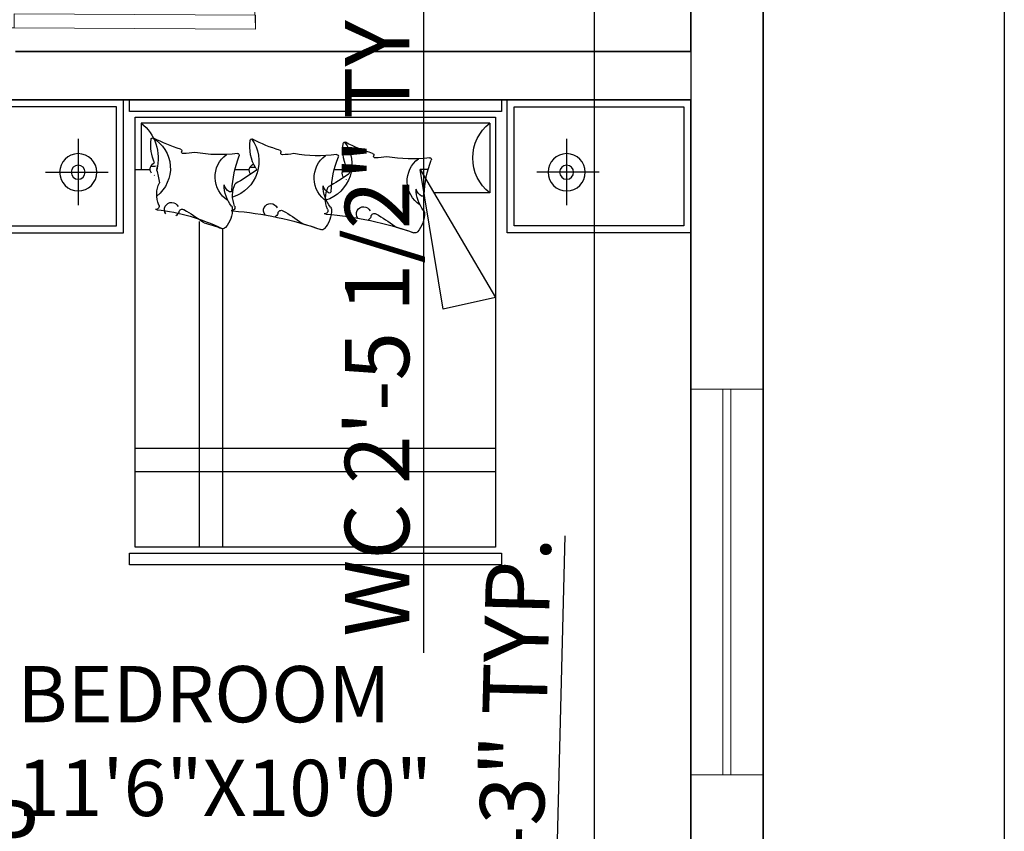
# Model space of a CAD drawing. Units: inches. Extents: x 3394 to 4794, y 965 to 1718.
# Tile 5 of 15: x 3818 to 3941, y 1237 to 1338. Entities that reach past the tile are written whole.
import ezdxf

# ---------------------------------------------------------------- set-up
doc = ezdxf.new("R2010")
doc.units = ezdxf.units.IN
for name, color, linetype, lineweight in [('A-ANNO-DIMS', 2, 'Continuous', 13), ('A-AREA-IDEN', 7, 'Continuous', 18), ('A-DOOR', 4, 'Continuous', 18), ('A-GLAZ', 4, 'Continuous', 18), ('A-WALL', 7, 'Continuous', 35), ('C-PROP', 7, 'Continuous', 25), ('NOITHAT', 21, 'Continuous', 18)]:
    doc.layers.add(name, color=color, linetype=linetype, lineweight=lineweight)
for name, color, linetype in [('FUR', 42, 'Continuous'), ('HA', 9, 'Continuous'), ('HID', 11, 'Continuous'), ('SAN', 5, 'Continuous')]:
    doc.layers.add(name, color=color, linetype=linetype)
doc.styles.get("Standard").update_dxf_attribs({"font": 'arial.ttf'})
doc.dimstyles.new('ISO-25', dxfattribs={"dimtxt": 8, "dimasz": 2.5, "dimexe": 1.25, "dimexo": 0.625, "dimtad": 1, "dimlunit": 3, "dimtxsty": 'Standard', "dimcen": 2.5, "dimadec": 0, "dimazin": 0, "dimtfac": 1, "dimtmove": 0, "dimatfit": 3, "dimfxl": 1, "dimarcsym": 0})

# ---------------------------------------------------------------- blocks, each defined once
blk = doc.blocks.new('*U5')
for p, q in [((0, 0), (0, -6)), ((30, 0), (30, -6))]:
    blk.add_line(p, q)
blk.add_lwpolyline([(0, 0), (0, 30), (1.75, 30), (1.75, 0)], close=True)
blk.add_arc((0, 0), 30, 0, 90)
blk = doc.blocks.new('A$C73A16738')
at = {"layer": 'FUR'}
for p, q in [((1.15, 2.3893), (1.1, 2.1643)), ((1.7, 2.0643), (1.15, 2.3893)), ((1.6, 2.3643), (1.6, 2.1234)), ((1.9, 2.3643), (1.6, 2.3643)), ((1.9, 2.3643), (1.9, 0.8643)), ((1.1, 2.1643), (1.7, 2.0643)), ((1.7, 2.099), (1.7, 2.0643)), ((1.7, 1.6955), (1.7, 1.7349)), ((1.7, 1.2682), (1.7, 1.3299)), ((1.7, 0.8393), (1.7, 0.9036)), ((1.9, 0.8643), (1.7, 0.8643))]:
    blk.add_line(p, q, dxfattribs=at)
for points in [[(1.428, 2.4393), (2, 2.4393), (2, 3.2287), (1.428, 3.2287)], [(1.458, 2.4693), (1.97, 2.4693), (1.97, 3.1987), (1.458, 3.1987)], [(0, 2.4143), (0, 0.8143), (0.05, 0.8143), (0.05, 2.4143)], [(1.95, 2.4143), (1.95, 0.8143), (2, 0.8143), (2, 2.4143)], [(0.075, 0.8393), (1.925, 0.8393), (1.925, 2.3893), (0.075, 2.3893)], [(1.428, 0.7893), (2, 0.7893), (2, 0), (1.428, 0)], [(1.458, 0.7593), (1.97, 0.7593), (1.97, 0.03), (1.458, 0.03)]]:
    blk.add_lwpolyline(points, close=True, dxfattribs=at)
for centre, start, end in [((1.75, 2.4806), 217.7826, 322.2174), ((1.75, 0.7481), 37.7826, 105.2747)]:
    blk.add_arc(centre, 0.1898, start, end, dxfattribs=at)
at = {"layer": 'HA'}
for p, q in [((0.4, 2.3893), (0.4, 0.8393)), ((0.5, 2.3893), (0.5, 0.8393)), ((1.4456, 1.2143), (0.075, 1.2143)), ((1.4772, 1.1143), (0.075, 1.1143))]:
    blk.add_line(p, q, dxfattribs=at)
at = {"layer": 'HID'}
for centre, radius, start, end in [((1.5102, 1.9654), 0.1174, 87.3377, 131.666), ((1.515, 2.0683), 0.0144, 51.6071, 87.3377), ((1.6169, 2.1969), 0.1496, 231.6071, 269.7845), ((1.5925, 2.0742), 0.0072, 92.7363, 208.2985), ((1.5692, 2.5605), 0.4796, 272.7363, 290.959), ((1.7434, 2.1059), 0.0072, 352.7248, 110.959), ((2.3483, 2.0286), 0.6026, 172.7248, 190.2702), ((1.4417, 2.0424), 0.0144, 131.666, 199.4465), ((0.016, 1.539), 1.4976, 4.5852, 19.4465), ((0.016, 1.539), 1.4976, 16.386, 19.4465), ((1.6496, 2.1284), 0.1197, 212.7628, 323.8922), ((1.628, 2.0933), 0.0475, 208.2985, 255.7891), ((1.4666, 1.9655), 0.0144, 196.386, 223.7955), ((0.9264, 1.5508), 0.6667, 29.049, 37.3823), ((2.0379, 1.8684), 0.2875, 169.4168, 179.3085), ((1.4966, 1.8675), 0.0144, 282.6426, 29.049), ((1.7576, 1.8718), 0.0072, 179.3085, 290.689), ((1.7627, 1.8583), 0.0072, 16.2196, 110.689), ((1.5097, 1.8233), 0.0319, 112.7015, 147.1556), ((1.5097, 1.8214), 0.0305, 232.3565, 65.7762), ((1.5029, 1.8394), 0.0144, 102.6426, 112.7015), ((2.3483, 2.0286), 0.6026, 196.2196, 208.2114), ((1.7225, 1.6087), 0.1623, 53.8947, 162.3952), ((2.8537, 0.9606), 1.4182, 145.8329, 150.0245), ((3.1426, 2.3695), 1.6108, 202.7018, 202.7206), ((1.6834, 1.7584), 0.0288, 232.662, 339.1573), ((1.6862, 1.7531), 0.0072, 38.8315, 145.8329), ((1.788, 1.9236), 0.1919, 239.9211, 277.124), ((0.088, 1.8308), 1.6108, 356.4982, 357.2888), ((1.8109, 1.7404), 0.0072, 277.124, 28.2114), ((1.8109, 1.7404), 0.0072, 277.124, 28.2114), ((1.5829, 2.1606), 0.4796, 272.7363, 290.959), ((1.7571, 1.706), 0.0072, 352.7248, 110.959), ((2.362, 1.6287), 0.6026, 172.7248, 190.2702), ((1.4554, 1.6425), 0.0144, 131.666, 199.4465), ((1.5239, 1.5655), 0.1174, 87.3377, 131.666), ((1.5236, 1.6535), 0.0144, 67.1663, 184.3422), ((1.5745, 1.7743), 0.1167, 247.1663, 295.7613), ((1.5287, 1.6684), 0.0144, 51.6071, 87.3377), ((1.6306, 1.797), 0.1496, 231.6071, 269.7845), ((1.6633, 1.7284), 0.1197, 212.7628, 323.8922), ((1.6062, 1.6743), 0.0072, 92.7363, 208.2985), ((1.6417, 1.6934), 0.0475, 208.2985, 255.7891), ((0.0297, 1.1391), 1.4976, 4.5852, 19.4465), ((0.0297, 1.1391), 1.4976, 16.386, 19.4465), ((1.4803, 1.5656), 0.0144, 196.386, 223.7955), ((0.9401, 1.1509), 0.6667, 29.049, 37.3823), ((2.0516, 1.4685), 0.2875, 169.4168, 179.3085), ((1.5234, 1.4234), 0.0319, 112.7015, 147.1556), ((1.5234, 1.4215), 0.0305, 232.3565, 65.7762), ((1.5166, 1.4395), 0.0144, 102.6426, 112.7015), ((1.5103, 1.4676), 0.0144, 282.6426, 29.049), ((1.7713, 1.4719), 0.0072, 179.3085, 290.689), ((1.7764, 1.4584), 0.0072, 16.2196, 110.689), ((2.362, 1.6287), 0.6026, 196.2196, 208.2114), ((1.7362, 1.2088), 0.1623, 53.8947, 162.3952), ((2.8674, 0.5607), 1.4182, 145.8329, 150.0245), ((1.6999, 1.3531), 0.0072, 38.8315, 145.8329), ((1.8017, 1.5237), 0.1919, 239.9211, 277.124), ((3.1563, 1.9695), 1.6108, 202.7018, 202.7206), ((1.6971, 1.3585), 0.0288, 232.662, 339.1573), ((0.1017, 1.4309), 1.6108, 356.4982, 357.2888), ((1.8246, 1.3404), 0.0072, 277.124, 28.2114), ((1.8246, 1.3404), 0.0072, 277.124, 28.2114), ((1.5877, 1.7344), 0.4796, 272.7363, 290.959), ((1.7618, 1.2798), 0.0072, 352.7248, 110.959), ((2.3667, 1.2026), 0.6026, 172.7248, 190.2702), ((1.5286, 1.1394), 0.1174, 87.3377, 131.666), ((1.5373, 1.2536), 0.0144, 67.1663, 184.3422), ((1.5334, 1.2423), 0.0144, 51.6071, 87.3377), ((1.6353, 1.3709), 0.1496, 231.6071, 269.7845), ((1.5882, 1.3744), 0.1167, 247.1663, 295.7613), ((1.6681, 1.3023), 0.1197, 212.7628, 323.8922), ((1.6109, 1.2482), 0.0072, 92.7363, 208.2985), ((1.6464, 1.2673), 0.0475, 208.2985, 255.7891), ((1.4601, 1.2163), 0.0144, 131.666, 199.4465), ((0.6883, 0.8412), 0.8439, 6.224, 26.0326), ((0.0344, 0.713), 1.4976, 16.386, 19.4465), ((1.485, 1.1395), 0.0144, 196.386, 223.7955), ((0.9449, 0.7248), 0.6667, 29.049, 37.3823), ((2.0564, 1.0424), 0.2875, 169.4168, 179.3085), ((1.5281, 0.9972), 0.0319, 112.7015, 147.1556), ((1.5282, 0.9954), 0.0305, 232.3565, 65.7762), ((1.5214, 1.0134), 0.0144, 102.6426, 112.7015), ((1.5151, 1.0415), 0.0144, 282.6426, 29.049), ((1.7761, 1.0457), 0.0072, 179.3085, 290.689), ((1.7812, 1.0323), 0.0072, 16.2196, 110.689), ((2.3667, 1.2026), 0.6026, 196.2196, 208.2114), ((1.7054, 0.84), 0.1504, 29.3598, 142.4281), ((1.5421, 0.9274), 0.0144, 67.1663, 184.3422), ((1.5929, 1.0482), 0.1167, 247.1663, 295.7613), ((1.5813, 0.5283), 0.4195, 73.7524, 81.4605), ((1.7047, 0.927), 0.0072, 38.8315, 145.8329), ((3.1611, 1.5434), 1.6108, 202.7018, 202.7206), ((1.7018, 0.9324), 0.0288, 232.662, 339.1573), ((0.1065, 1.0048), 1.6108, 356.4982, 357.2888), ((1.8064, 1.0976), 0.1919, 246.1093, 277.124), ((1.8293, 0.9143), 0.0072, 277.124, 28.2114), ((1.8293, 0.9143), 0.0072, 277.124, 28.2114)]:
    blk.add_arc(centre, radius, start, end, dxfattribs=at)
at = {"layer": 'SAN'}
for p, q in [((1.6885, 2.8351), (1.6885, 2.5658)), ((1.8316, 2.6947), (1.5465, 2.6947)), ((1.6885, 0.4536), (1.6885, 0.7229)), ((1.8316, 0.594), (1.5465, 0.594))]:
    blk.add_line(p, q, dxfattribs=at)
for centre, radius in [((1.6885, 2.6947), 0.08), ((1.6885, 2.6947), 0.03), ((1.6885, 0.594), 0.08), ((1.6885, 0.594), 0.03)]:
    blk.add_circle(centre, radius, dxfattribs=at)
blk = doc.blocks.new('WIN-48IN')
for p, q in [((9, 48), (0, 48)), ((4, 0), (4, 48)), ((5, 0), (5, 48)), ((9, 0), (0, 0))]:
    blk.add_line(p, q)
blk = doc.blocks.new('*D80')
at = {"layer": 'A-ANNO-DIMS', "color": 0, "lineweight": -2, "transparency": 16777216}
for p, q in [((3872.33, 1381.68), (3867.26, 1381.68)), ((3868.51, 1379.18), (3868.51, 1354.58)), ((3872.33, 1352.08), (3867.26, 1352.08)), ((3868.51, 1352.08), (3868.51, 1258.87))]:
    blk.add_line(p, q, dxfattribs=at)
at = {"layer": 'A-ANNO-DIMS', "color": 0, "transparency": 16777216}
for points in [[(3868.09, 1379.18), (3868.93, 1379.18), (3868.51, 1381.68)], [(3868.09, 1354.58), (3868.93, 1354.58), (3868.51, 1352.08)]]:
    blk.add_solid(points, dxfattribs=at)
at = {"layer": 'Defpoints', "color": 0, "transparency": 16777216}
for p in [(3872.95, 1381.68), (3868.51, 1352.08), (3872.95, 1352.08)]:
    blk.add_point(p, dxfattribs=at)
at = {"layer": 'A-ANNO-DIMS', "color": 0, "transparency": 16777216, "insert": (3863.75, 1304.22), "char_height": 8, "attachment_point": 5, "rotation": 90}
blk.add_mtext('WC 2\'-5 1/2" TYP.', dxfattribs=at)
blk = doc.blocks.new('*D84')
at = {"layer": 'A-ANNO-DIMS', "color": 0, "lineweight": -2, "transparency": 16777216}
for p, q in [((3828.32, 1230.52), (3710.44, 1233.52)), ((3828.15, 1223.75), (3828.35, 1231.77)), ((3875.11, 1229.33), (3830.82, 1230.46)), ((3877.44, 1222.5), (3877.64, 1230.51))]:
    blk.add_line(p, q, dxfattribs=at)
at = {"layer": 'A-ANNO-DIMS', "color": 0, "transparency": 16777216}
for points in [[(3830.83, 1230.87), (3830.81, 1230.04), (3828.32, 1230.52)], [(3875.12, 1229.75), (3875.1, 1228.91), (3877.61, 1229.27)]]:
    blk.add_solid(points, dxfattribs=at)
at = {"layer": 'Defpoints', "color": 0, "transparency": 16777216}
for p in [(3828.32, 1230.52), (3828.13, 1223.13), (3877.42, 1221.87)]:
    blk.add_point(p, dxfattribs=at)
at = {"layer": 'A-ANNO-DIMS', "color": 0, "transparency": 16777216, "insert": (3768.25, 1236.81), "char_height": 8, "attachment_point": 5, "rotation": 358.5431}
blk.add_mtext('TV UNIT 4\'-1 1/2" TYP.', dxfattribs=at)
blk = doc.blocks.new('*D85')
at = {"layer": 'A-ANNO-DIMS', "color": 0, "lineweight": -2, "transparency": 16777216}
for p, q in [((3884.82, 1221.68), (3886.13, 1273.43)), ((3878.05, 1221.86), (3886.06, 1221.65)), ((3884.5, 1209.23), (3884.75, 1219.18)), ((3877.67, 1206.91), (3885.68, 1206.7))]:
    blk.add_line(p, q, dxfattribs=at)
at = {"layer": 'A-ANNO-DIMS', "color": 0, "transparency": 16777216}
for points in [[(3884.33, 1219.2), (3885.17, 1219.17), (3884.82, 1221.68)], [(3884.08, 1209.24), (3884.91, 1209.22), (3884.43, 1206.73)]]:
    blk.add_solid(points, dxfattribs=at)
at = {"layer": 'Defpoints', "color": 0, "transparency": 16777216}
for p in [(3877.42, 1221.87), (3884.82, 1221.68), (3877.04, 1206.92)]:
    blk.add_point(p, dxfattribs=at)
at = {"layer": 'A-ANNO-DIMS', "color": 0, "transparency": 16777216, "insert": (3880.79, 1248.93), "char_height": 8, "attachment_point": 5, "rotation": 88.5431}
blk.add_mtext('1\'-3" TYP.', dxfattribs=at)
blk = doc.blocks.new('*D125')
at = {"layer": 'A-ANNO-DIMS', "color": 0, "lineweight": -2, "transparency": 16777216}
for p, q in [((3889.74, 1381.06), (3889.74, 987.36)), ((3901.74, 1381.06), (3901.74, 987.36)), ((3892.24, 988.61), (3899.24, 988.61)), ((3901.74, 988.61), (3926.01, 988.61))]:
    blk.add_line(p, q, dxfattribs=at)
at = {"layer": 'A-ANNO-DIMS', "color": 0, "transparency": 16777216}
for points in [[(3892.24, 989.03), (3892.24, 988.2), (3889.74, 988.61)], [(3899.24, 989.03), (3899.24, 988.2), (3901.74, 988.61)]]:
    blk.add_solid(points, dxfattribs=at)
at = {"layer": 'Defpoints', "color": 0, "transparency": 16777216}
for p in [(3889.74, 1381.68), (3901.74, 1381.68), (3901.74, 988.61)]:
    blk.add_point(p, dxfattribs=at)
at = {"layer": 'A-ANNO-DIMS', "color": 0, "transparency": 16777216, "insert": (3915.13, 993.32), "char_height": 8, "attachment_point": 5}
blk.add_mtext('1\'-0"', dxfattribs=at)

msp = doc.modelspace()

# ---------------------------------------------------------------- linework, layer by layer
at = {"layer": 'A-WALL'}
for p, q in [((3910.745, 1582.682), (3910.745, 1198.682)), ((3901.745, 1381.682), (3901.745, 1333.682)), ((3817.745, 1333.682), (3901.745, 1333.682)), ((3802.745, 1327.682), (3901.745, 1327.682)), ((3901.745, 1327.682), (3901.745, 1207.682))]:
    msp.add_line(p, q, dxfattribs=at)
at = {"layer": 'C-PROP'}
msp.add_line((3940.745, 1666.682), (3940.745, 1057.682), dxfattribs=at)

# ---------------------------------------------------------------- block references
at = {"layer": 'A-DOOR', "xscale": -1, "rotation": 269.6786649249897}
msp.add_blockref('*U5', (3817.576, 1336.649), dxfattribs=at)
at = {"layer": 'A-GLAZ'}
msp.add_blockref('WIN-48IN', (3901.745, 1243.682), dxfattribs=at)
at = {"layer": 'NOITHAT', "xscale": -28.92215291203286, "yscale": 28.92215291203286, "zscale": 28.92215291203286, "rotation": 270}
msp.add_blockref('A$C73A16738', (3808.364, 1269.838), dxfattribs=at)

# ---------------------------------------------------------------- texts
at = {"layer": 'A-AREA-IDEN', "insert": (3817.939, 1257.24), "char_height": 7, "attachment_point": 1}
msp.add_mtext_dynamic_manual_height_columns('{\\fTimes New Roman|b0|i0|c0|p18;BEDROOM\\P11\'6"X10\'0"}', width=61.05572, gutter_width=12.5, heights=[0], dxfattribs=at)

# ---------------------------------------------------------------- dimensions: what is measured, and where the dimension line sits
at = {"layer": 'A-ANNO-DIMS'}
for base, p1, p2, angle, text, picture, middle in [((3868.511, 1352.075), (3872.953, 1381.682), (3872.953, 1352.075), 270, 'WC <> TYP.', '*D80', (3863.75, 1304.222)), ((3884.815, 1221.684), (3877.042, 1206.923), (3877.422, 1221.872), 88.54308, '<> TYP.', '*D85', (3880.794, 1248.925)), ((3828.323, 1230.519), (3877.422, 1221.872), (3828.135, 1223.125), 178.54308, 'TV UNIT <> TYP.', '*D84', (3768.252, 1236.809))]:
    dim = msp.add_linear_dim(base=base, p1=p1, p2=p2, angle=angle, text=text, dimstyle='ISO-25', override={"dimdec": 1, "dimlfac": 1, "dimrnd": 0, "dimzin": 1, "dimdsep": 46, "dimlunit": 4, "dimfrac": 2}, dxfattribs=at)
    dim.commit()
    dim.dimension.update_dxf_attribs({"geometry": picture, "text_midpoint": middle})
dim = msp.add_linear_dim(base=(3901.745, 988.612), p1=(3889.745, 1381.682), p2=(3901.745, 1381.682), dimstyle='ISO-25', override={"dimdec": 1, "dimlfac": 1, "dimrnd": 0, "dimzin": 1, "dimdsep": 46, "dimlunit": 4, "dimfrac": 2}, dxfattribs=at)
dim.commit()
dim.dimension.update_dxf_attribs({"geometry": '*D125', "text_midpoint": (3915.126, 993.322)})

doc.saveas('drawing.dxf')
